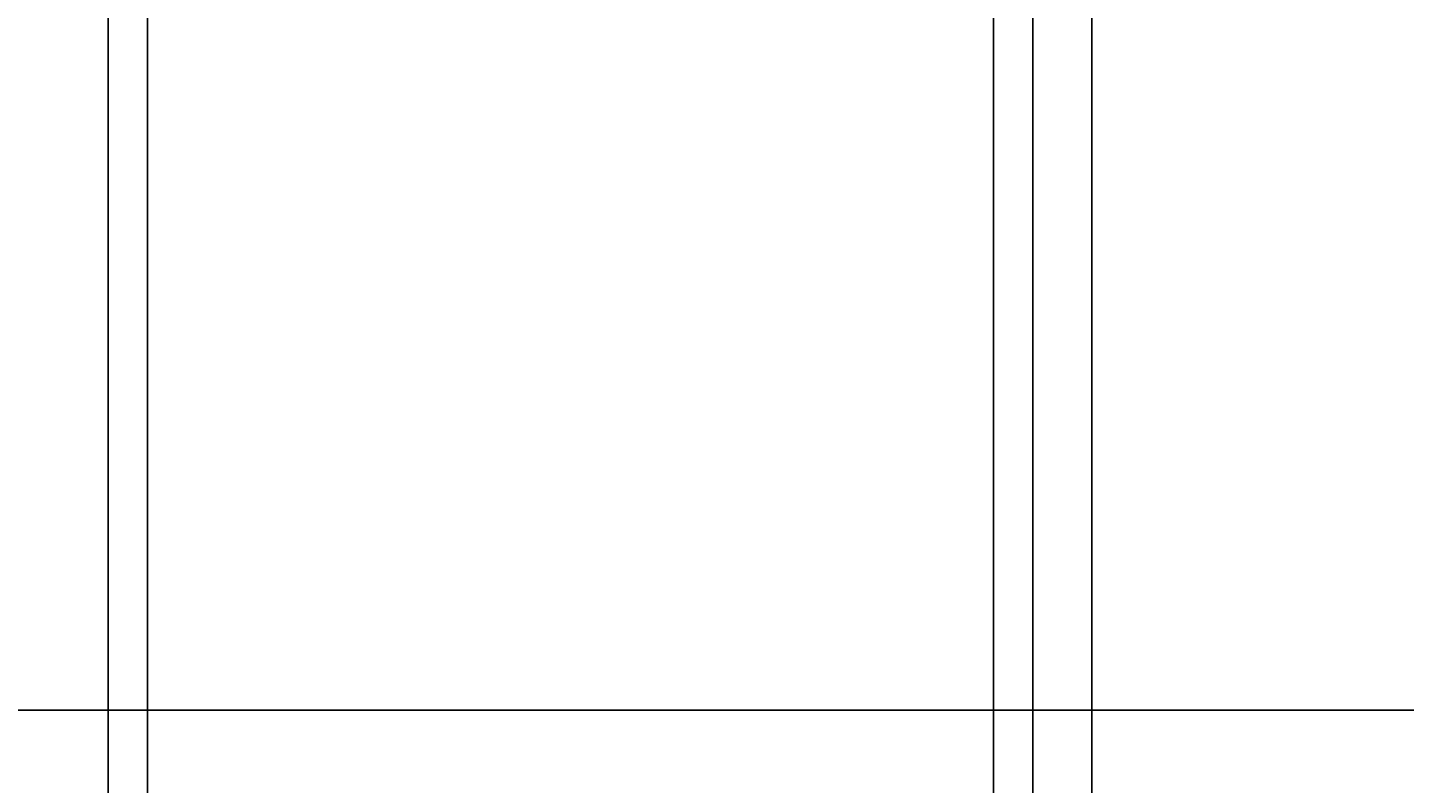
# Model space of a CAD drawing. Units: inches. Extents: x -6 to 289, y -8 to 323.
# Tile 34 of 107: x 209 to 244, y 49 to 68. Entities that reach past the tile are written whole.
import ezdxf

# ---------------------------------------------------------------- set-up
doc = ezdxf.new("R2010")
doc.units = ezdxf.units.IN
doc.header["$MEASUREMENT"] = 0
doc.layers.add('A-ANNO-DIMS', color=2, linetype='Continuous', lineweight=18)
doc.layers.add('A-DOOR', color=3, linetype='Continuous', lineweight=25)
doc.styles.get("Standard").update_dxf_attribs({"font": 'arial.ttf'})
doc.dimstyles.get("Standard").update_dxf_attribs({"dimtxt": 0.18, "dimasz": 0.18, "dimexe": 0.18, "dimexo": 0.0625, "dimgap": 0.09, "dimtad": 0, "dimtih": 1, "dimtoh": 1, "dimdec": 4, "dimzin": 0, "dimdsep": 46, "dimtxsty": 'Standard', "dimcen": 0.09, "dimadec": 0, "dimazin": 0, "dimtfac": 1, "dimtdec": 4, "dimtofl": 0, "dimtmove": 0, "dimatfit": 3, "dimfxl": 1, "dimtolj": 1, "dimtzin": 0, "dimarcsym": 0})

# ---------------------------------------------------------------- blocks, each defined once
blk = doc.blocks.new('*D16')
at = {"layer": 'A-ANNO-DIMS', "color": 0, "lineweight": -2, "transparency": 16777216}
for p, q in [((9.943, 68.37), (9.943, -8.391)), ((272.973, 68.37), (272.973, -8.391)), ((10.123, -8.211), (140.993, -8.211)), ((272.793, -8.211), (141.923, -8.211))]:
    blk.add_line(p, q, dxfattribs=at)
at = {"layer": 'A-ANNO-DIMS', "color": 0, "transparency": 16777216}
for points in [[(10.123, -8.181), (10.123, -8.241), (9.943, -8.211)], [(272.793, -8.181), (272.793, -8.241), (272.973, -8.211)]]:
    blk.add_solid(points, dxfattribs=at)
at = {"layer": 'Defpoints', "color": 0, "transparency": 16777216}
for p in [(9.943, 68.432), (272.973, 68.432), (272.973, -8.211)]:
    blk.add_point(p, dxfattribs=at)
at = {"layer": 'A-ANNO-DIMS', "color": 0, "transparency": 16777216, "insert": (141.458, -8.211), "char_height": 0.18, "attachment_point": 5}
blk.add_mtext('\\A1;263.03', dxfattribs=at)
blk = doc.blocks.new('*D42')
at = {"layer": 'A-ANNO-DIMS', "color": 0, "lineweight": -2, "transparency": 16777216}
for p, q in [((190.792, 224.326), (190.792, -8.391)), ((211.292, 224.326), (211.292, -8.391)), ((190.972, -8.211), (200.716, -8.211)), ((211.112, -8.211), (201.368, -8.211))]:
    blk.add_line(p, q, dxfattribs=at)
at = {"layer": 'A-ANNO-DIMS', "color": 0, "transparency": 16777216}
for points in [[(190.972, -8.181), (190.972, -8.241), (190.792, -8.211)], [(211.112, -8.181), (211.112, -8.241), (211.292, -8.211)]]:
    blk.add_solid(points, dxfattribs=at)
at = {"layer": 'Defpoints', "color": 0, "transparency": 16777216}
for p in [(190.792, 224.389), (211.292, 224.389), (211.292, -8.211)]:
    blk.add_point(p, dxfattribs=at)
at = {"layer": 'A-ANNO-DIMS', "color": 0, "transparency": 16777216, "insert": (201.042, -8.211), "char_height": 0.18, "attachment_point": 5}
blk.add_mtext('\\A1;20.5', dxfattribs=at)
blk = doc.blocks.new('*D43')
at = {"layer": 'A-ANNO-DIMS', "color": 0, "lineweight": -2, "transparency": 16777216}
for p, q in [((211.292, 224.326), (211.292, -8.391)), ((212.292, 224.326), (212.292, -8.391)), ((211.472, -8.211), (211.669, -8.211)), ((212.112, -8.211), (211.915, -8.211))]:
    blk.add_line(p, q, dxfattribs=at)
at = {"layer": 'A-ANNO-DIMS', "color": 0, "transparency": 16777216}
for points in [[(211.472, -8.181), (211.472, -8.241), (211.292, -8.211)], [(212.112, -8.181), (212.112, -8.241), (212.292, -8.211)]]:
    blk.add_solid(points, dxfattribs=at)
at = {"layer": 'Defpoints', "color": 0, "transparency": 16777216}
for p in [(211.292, 224.389), (212.292, 224.389), (212.292, -8.211)]:
    blk.add_point(p, dxfattribs=at)
at = {"layer": 'A-ANNO-DIMS', "color": 0, "transparency": 16777216, "insert": (211.792, -8.211), "char_height": 0.18, "attachment_point": 5}
blk.add_mtext('\\A1;1', dxfattribs=at)
blk = doc.blocks.new('*D44')
at = {"layer": 'A-ANNO-DIMS', "color": 0, "lineweight": -2, "transparency": 16777216}
for p, q in [((212.292, 224.326), (212.292, -8.391)), ((233.792, 224.326), (233.792, -8.391)), ((212.472, -8.211), (222.716, -8.211)), ((233.612, -8.211), (223.368, -8.211))]:
    blk.add_line(p, q, dxfattribs=at)
at = {"layer": 'A-ANNO-DIMS', "color": 0, "transparency": 16777216}
for points in [[(212.472, -8.181), (212.472, -8.241), (212.292, -8.211)], [(233.612, -8.181), (233.612, -8.241), (233.792, -8.211)]]:
    blk.add_solid(points, dxfattribs=at)
at = {"layer": 'Defpoints', "color": 0, "transparency": 16777216}
for p in [(212.292, 224.389), (233.792, 224.389), (233.792, -8.211)]:
    blk.add_point(p, dxfattribs=at)
at = {"layer": 'A-ANNO-DIMS', "color": 0, "transparency": 16777216, "insert": (223.042, -8.211), "char_height": 0.18, "attachment_point": 5}
blk.add_mtext('\\A1;21.5', dxfattribs=at)
blk = doc.blocks.new('*D45')
at = {"layer": 'A-ANNO-DIMS', "color": 0, "lineweight": -2, "transparency": 16777216}
for p, q in [((234.792, 225.326), (234.792, -8.391)), ((233.792, 224.326), (233.792, -8.391)), ((233.972, -8.211), (234.169, -8.211)), ((234.612, -8.211), (234.415, -8.211))]:
    blk.add_line(p, q, dxfattribs=at)
at = {"layer": 'A-ANNO-DIMS', "color": 0, "transparency": 16777216}
for points in [[(233.972, -8.181), (233.972, -8.241), (233.792, -8.211)], [(234.612, -8.181), (234.612, -8.241), (234.792, -8.211)]]:
    blk.add_solid(points, dxfattribs=at)
at = {"layer": 'Defpoints', "color": 0, "transparency": 16777216}
for p in [(234.792, 225.389), (233.792, 224.389), (234.792, -8.211)]:
    blk.add_point(p, dxfattribs=at)
at = {"layer": 'A-ANNO-DIMS', "color": 0, "transparency": 16777216, "insert": (234.292, -8.211), "char_height": 0.18, "attachment_point": 5}
blk.add_mtext('\\A1;1', dxfattribs=at)
blk = doc.blocks.new('*D46')
at = {"layer": 'A-ANNO-DIMS', "color": 0, "lineweight": -2, "transparency": 16777216}
for p, q in [((236.292, 226.826), (236.292, -8.391)), ((234.792, 225.326), (234.792, -8.391)), ((234.972, -8.211), (235.296, -8.211)), ((236.112, -8.211), (235.788, -8.211))]:
    blk.add_line(p, q, dxfattribs=at)
at = {"layer": 'A-ANNO-DIMS', "color": 0, "transparency": 16777216}
for points in [[(234.972, -8.181), (234.972, -8.241), (234.792, -8.211)], [(236.112, -8.181), (236.112, -8.241), (236.292, -8.211)]]:
    blk.add_solid(points, dxfattribs=at)
at = {"layer": 'Defpoints', "color": 0, "transparency": 16777216}
for p in [(236.292, 226.889), (234.792, 225.389), (236.292, -8.211)]:
    blk.add_point(p, dxfattribs=at)
at = {"layer": 'A-ANNO-DIMS', "color": 0, "transparency": 16777216, "insert": (235.542, -8.211), "char_height": 0.18, "attachment_point": 5}
blk.add_mtext('\\A1;1.5', dxfattribs=at)
blk = doc.blocks.new('*D81')
at = {"layer": 'A-ANNO-DIMS', "color": 0, "lineweight": -2, "transparency": 16777216}
for p, q in [((230.292, 68.842), (230.292, 322.969)), ((230.472, 322.789), (237.298, 322.789)), ((245.035, 322.789), (238.208, 322.789)), ((245.215, 66.286), (245.215, 322.969))]:
    blk.add_line(p, q, dxfattribs=at)
at = {"layer": 'A-ANNO-DIMS', "color": 0, "transparency": 16777216}
for points in [[(230.472, 322.819), (230.472, 322.759), (230.292, 322.789)], [(245.035, 322.819), (245.035, 322.759), (245.215, 322.789)]]:
    blk.add_solid(points, dxfattribs=at)
at = {"layer": 'Defpoints', "color": 0, "transparency": 16777216}
for p in [(245.215, 322.789), (230.292, 68.779), (245.215, 66.224)]:
    blk.add_point(p, dxfattribs=at)
at = {"layer": 'A-ANNO-DIMS', "color": 0, "transparency": 16777216, "insert": (237.753, 322.789), "char_height": 0.18, "attachment_point": 5}
blk.add_mtext('\\A1;14.923', dxfattribs=at)
blk = doc.blocks.new('*D90')
at = {"layer": 'A-ANNO-DIMS', "color": 0, "lineweight": -2, "transparency": 16777216}
for p, q in [((230.354, 68.779), (288.653, 68.779)), ((288.473, 68.599), (288.473, 60.114)), ((288.473, 51.265), (288.473, 59.75)), ((247.303, 51.085), (288.653, 51.085))]:
    blk.add_line(p, q, dxfattribs=at)
at = {"layer": 'A-ANNO-DIMS', "color": 0, "transparency": 16777216}
for points in [[(288.443, 68.599), (288.503, 68.599), (288.473, 68.779)], [(288.443, 51.265), (288.503, 51.265), (288.473, 51.085)]]:
    blk.add_solid(points, dxfattribs=at)
at = {"layer": 'Defpoints', "color": 0, "transparency": 16777216}
for p in [(230.292, 68.779), (288.473, 68.779), (247.241, 51.085)]:
    blk.add_point(p, dxfattribs=at)
at = {"layer": 'A-ANNO-DIMS', "color": 0, "transparency": 16777216, "insert": (288.473, 59.932), "char_height": 0.18, "attachment_point": 5}
blk.add_mtext('\\A1;17.694', dxfattribs=at)

msp = doc.modelspace()

# ---------------------------------------------------------------- linework, layer by layer
at = {"layer": 'A-DOOR'}
msp.add_lwpolyline([(121.008, 51.0851), (247.2408, 51.0851), (247.2408, 7.2888), (121.008, 7.2888)], close=True, dxfattribs=at)

# ---------------------------------------------------------------- dimensions: what is measured, and where the dimension line sits
at = {"layer": 'A-ANNO-DIMS'}
for base, p1, p2, override, picture, middle in [((245.2146, 322.7888), (230.2918, 68.7795), (245.2146, 66.2238), {"dimdec": 3, "dimlfac": 1, "dimrnd": 0, "dimzin": 0, "dimdsep": 46, "dimlunit": 2}, '*D81', (237.7532, 322.7888)), ((236.2918, -8.2112), (234.7918, 225.3887), (236.2918, 226.8887), {"dimdec": 1, "dimlfac": 1, "dimrnd": 0, "dimzin": 0, "dimdsep": 46, "dimlunit": 2}, '*D46', (235.5418, -8.2112)), ((234.7918, -8.2112), (233.7918, 224.3887), (234.7918, 225.3887), {"dimdec": 0, "dimlfac": 1, "dimrnd": 0, "dimzin": 0, "dimdsep": 46, "dimlunit": 2}, '*D45', (234.2918, -8.2112)), ((211.2918, -8.2112), (190.7918, 224.3887), (211.2918, 224.3887), {"dimdec": 1, "dimlfac": 1, "dimrnd": 0, "dimzin": 0, "dimdsep": 46, "dimlunit": 2}, '*D42', (201.0418, -8.2112)), ((212.2918, -8.2112), (211.2918, 224.3887), (212.2918, 224.3887), {"dimdec": 0, "dimlfac": 1, "dimrnd": 0, "dimzin": 0, "dimdsep": 46, "dimlunit": 2}, '*D43', (211.7918, -8.2112)), ((233.7918, -8.2112), (212.2918, 224.3887), (233.7918, 224.3887), {"dimdec": 1, "dimlfac": 1, "dimrnd": 0, "dimzin": 0, "dimdsep": 46, "dimlunit": 2}, '*D44', (223.0418, -8.2112)), ((272.9733, -8.2112), (9.943, 68.4322), (272.9733, 68.4322), {"dimdec": 2, "dimlfac": 1, "dimrnd": 0, "dimzin": 0, "dimdsep": 46, "dimlunit": 2}, '*D16', (141.4581, -8.2112))]:
    dim = msp.add_linear_dim(base=base, p1=p1, p2=p2, dimstyle='Standard', override=override, dxfattribs=at)
    dim.commit()
    dim.dimension.update_dxf_attribs({"geometry": picture, "text_midpoint": middle})
dim = msp.add_linear_dim(base=(288.4733, 68.7795), p1=(247.2408, 51.0851), p2=(230.2918, 68.7795), angle=90, dimstyle='Standard', override={"dimdec": 3, "dimlfac": 1, "dimrnd": 0, "dimzin": 0, "dimdsep": 46, "dimlunit": 2}, dxfattribs=at)
dim.commit()
dim.dimension.update_dxf_attribs({"geometry": '*D90', "text_midpoint": (288.4733, 59.9323)})

doc.saveas('drawing.dxf')
